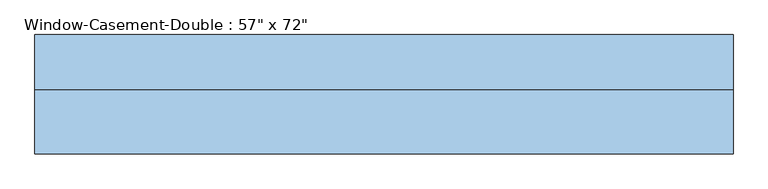
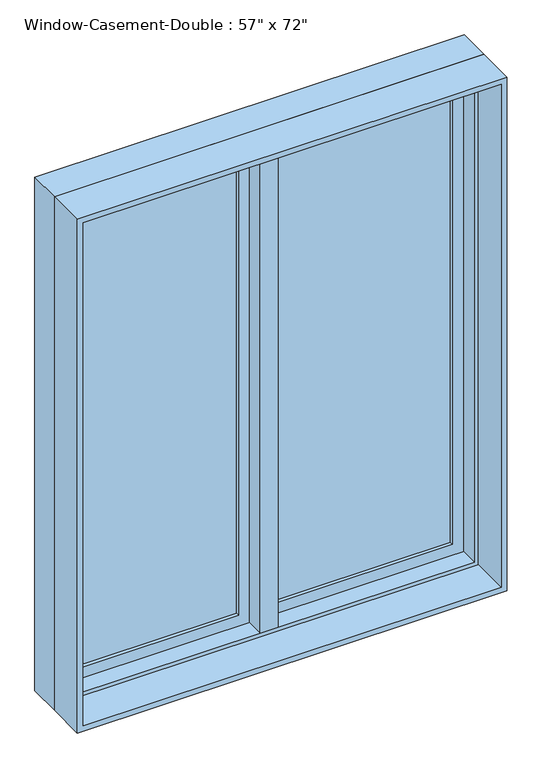
"""IFC4 building model written with IfcOpenShell, lengths in millimetres: window geometry."""

from ifc_helpers import new_model, si_unit, frame, origin, place, context, project, spatial, polyline, outline, extrude, faceted_brep, source, transform, mapped, element, save


def window_9ac97e1a(model_context):
    return source(origin(), model_context, "Body", "SolidModel", [
        faceted_brep([(9.525, 133.35, 2730.5), (-9.525, 133.35, 2730.5), (-9.525, 82.55, 2730.5), (9.525, 82.55, 2730.5), (9.525, 133.35, 927.1), (9.525, 82.55, 927.1), (-9.525, 82.55, 927.1), (-9.525, 133.35, 927.1), (-9.525, 82.55, 946.15), (-9.525, 82.55, 2711.45), (-30.1625, 82.55, 946.15), (-30.1625, 82.55, 2711.45), (-30.1625, 19.05, 946.15), (-30.1625, 19.05, 2711.45), (30.1625, 19.05, 946.15), (30.1625, 19.05, 2711.45), (30.1625, 82.55, 946.15), (30.1625, 82.55, 2711.45), (9.525, 82.55, 946.15), (9.525, 82.55, 2711.45)], [[[0, 1, 2, 3]], [[4, 5, 6, 7]], [[1, 0, 4, 7]], [[2, 1, 7, 6, 8, 9]], [[9, 8, 10, 11]], [[11, 10, 12, 13]], [[13, 12, 14, 15]], [[15, 14, 16, 17]], [[17, 16, 18, 19]], [[0, 3, 19, 18, 5, 4]], [[18, 8, 6, 5]], [[9, 19, 3, 2]], [[8, 18, 16, 14, 12, 10]], [[19, 9, 11, 13, 15, 17]]]),
        extrude(outline(polyline([(-66.675, 114.3), (-66.675, 107.95), (-654.05, 107.95), (-654.05, 114.3), (-66.675, 114.3)])), frame((0.0, 0.0, 984.25), z_axis=(0.0, 0.0, 1.0), x_axis=(1.0, 0.0, 0.0)), (0.0, 0.0, 1.0), 1689.1),
        extrude(outline(polyline([(-654.05, 95.25), (-654.05, 101.6), (-66.675, 101.6), (-66.675, 95.25), (-654.05, 95.25)])), frame((0.0, 0.0, 984.25), z_axis=(0.0, 0.0, 1.0), x_axis=(1.0, 0.0, 0.0)), (0.0, 0.0, 1.0), 1689.1),
        extrude(outline(polyline([(654.05, 114.3), (654.05, 107.95), (66.675, 107.95), (66.675, 114.3), (654.05, 114.3)])), frame((0.0, 0.0, 984.25), z_axis=(0.0, 0.0, 1.0), x_axis=(1.0, 0.0, 0.0)), (0.0, 0.0, 1.0), 1689.1),
        extrude(outline(polyline([(66.675, 95.25), (66.675, 101.6), (654.05, 101.6), (654.05, 95.25), (66.675, 95.25)])), frame((0.0, 0.0, 984.25), z_axis=(0.0, 0.0, 1.0), x_axis=(1.0, 0.0, 0.0)), (0.0, 0.0, 1.0), 1689.1),
        extrude(outline(polyline([(2730.5, -711.2), (927.1, -711.2), (927.1, -9.525), (2730.5, -9.525), (2730.5, -711.2)]), holes=[polyline([(2673.35, -66.675), (984.25, -66.675), (984.25, -654.05), (2673.35, -654.05), (2673.35, -66.675)])]), frame((0.0, 82.55, 0.0), z_axis=(0.0, 1.0, 0.0), x_axis=(0.0, 0.0, 1.0)), (0.0, 0.0, 1.0), 44.45),
        extrude(outline(polyline([(927.1, 711.2), (2730.5, 711.2), (2730.5, 9.525), (927.1, 9.525), (927.1, 711.2)]), holes=[polyline([(984.25, 66.675), (2673.35, 66.675), (2673.35, 654.05), (984.25, 654.05), (984.25, 66.675)])]), frame((0.0, 82.55, 0.0), z_axis=(0.0, 1.0, 0.0), x_axis=(0.0, 0.0, 1.0)), (0.0, 0.0, 1.0), 44.45),
        extrude(outline(polyline([(2743.2, -723.9), (914.4, -723.9), (914.4, 723.9), (2743.2, 723.9), (2743.2, -723.9)]), holes=[polyline([(2724.15, 704.85), (933.45, 704.85), (933.45, -704.85), (2724.15, -704.85), (2724.15, 704.85)])]), frame((0.0, -114.3, 0.0), z_axis=(0.0, 1.0, 0.0), x_axis=(0.0, 0.0, 1.0)), (0.0, 0.0, 1.0), 133.35),
        faceted_brep([(692.15, 82.55, 2711.45), (692.15, 19.05, 2711.45), (-692.15, 19.05, 2711.45), (-692.15, 82.55, 2711.45), (711.2, 133.35, 2730.5), (711.2, 82.55, 2730.5), (-711.2, 82.55, 2730.5), (-711.2, 133.35, 2730.5), (723.9, 19.05, 2743.2), (723.9, 133.35, 2743.2), (-723.9, 133.35, 2743.2), (-723.9, 19.05, 2743.2), (-692.15, 19.05, 946.15), (-692.15, 82.55, 946.15), (-711.2, 82.55, 927.1), (-711.2, 133.35, 927.1), (-723.9, 133.35, 914.4), (-723.9, 19.05, 914.4), (692.15, 19.05, 946.15), (692.15, 82.55, 946.15), (711.2, 82.55, 927.1), (711.2, 133.35, 927.1), (723.9, 133.35, 914.4), (723.9, 19.05, 914.4)], [[[0, 1, 2, 3]], [[4, 5, 6, 7]], [[8, 9, 10, 11]], [[3, 2, 12, 13]], [[7, 6, 14, 15]], [[11, 10, 16, 17]], [[13, 12, 18, 19]], [[15, 14, 20, 21]], [[17, 16, 22, 23]], [[11, 17, 23, 8], [1, 18, 12, 2]], [[19, 18, 1, 0]], [[5, 20, 14, 6], [3, 13, 19, 0]], [[21, 20, 5, 4]], [[23, 22, 9, 8]], [[9, 22, 16, 10], [7, 15, 21, 4]]]),
    ])


if __name__ == "__main__":
    model = new_model("IFC4")
    model_context = context("Model", 3, world=origin())
    ifc_project = project(units=[si_unit("LENGTHUNIT", "METRE", prefix="MILLI")], contexts=[model_context])
    site = spatial("IfcSite", under=ifc_project)
    building = spatial("IfcBuilding", under=site)
    placement = place(None, origin())
    window_shape = window_9ac97e1a(model_context)
    element("IfcWindow", 1, ObjectType="Window-Casement-Double : 57\" x 72\"", at=placement, inside=building, context=model_context, shape_type="MappedRepresentation", body=[
        mapped(window_shape, transform((0.0, 0.0, 0.0), x_axis=(1.0, 0.0, 0.0), y_axis=(0.0, 1.0, 0.0), z_axis=(0.0, 0.0, 1.0))),
    ])
    save(model, "model.ifc")

# Revit data of these elements
# Type "Window-Casement-Double : 57\" x 72\""
#   Type Mark = "17"
#   Fire Rating = "0.5h"
#   Assembly Code = "B2020100"
#   Analytic Construction = "Double glazing - domestic"
#   Frame Extension [instance default] = 0' - 0 1/4"
#   Window Inset [instance default] = 0' - 0"
#   Wall Thickness [instance default] = 0' - 6"
#   Interior Wall Closure [instance default] = 0' - 2 1/4"
#   Half Width = 2' - 4 1/2"
#   Visual Light Transmittance = 0.81
#   Thermal Resistance (R) = 1.8146 (h·ft²·°F)/BTU
#   Solar Heat Gain Coefficient = 0.76
#   Rough Width = 4' - 9 1/2"
#   Rough Height = 6' - 0 1/2"
#   Height = 6' - 0"
#   Heat Transfer Coefficient (U) = 0.5511 BTU/(h·ft²·°F)
#   Exterior Wall Closure [instance default] = 0' - 1 1/4"
#   Extension Jamb [instance default] = 0' - 2 1/4"
#   Default Sill Height = 3' - 0"
#   Width = 4' - 9"
#   Define Thermal Properties by = 0
#   Muntin Visibility = yes
#   Interior Trim Visibility [instance default] = yes
#   Exterior Trim Visibility [instance default] = yes
#   Extension Jamb Visibility [instance default] = yes
#   Interior Trim Material = Wood - Stained
#   Muntin Pattern = Muntin Pattern_2x2 : Muntin Pattern_2x2
#   Interior Trim = Trim-Window-Interior-Flat : Picture Frame
#   Interior Frame Material = Wood - Stained
#   Glass Panel Material = Glass
#   Exterior Trim Material = Clad - White
#   Exterior Trim = Trim-Window-Exterior-Flat : with Sill
#   Exterior Frame Material = Clad - White
#   Wall Closure = (empty or 0)
# Element 1 (IfcWindow, "Window-Casement-Double : 57\" x 72\"")
#   Wall Thickness = 0' - 9"
#   Extension Jamb = 0' - 5 1/4"
#   Materials on its faces: "Wood - Stained", "Glass", "Clad - White"
# Materials
#   "Wood - Stained": class "Wood", colour RGB 224 178 126, transparency 0, Cost = 0
#   "Glass": class "Glass", colour RGB 0 128 192, transparency 0.75, Description = "Soda Lime Glass", Cost = 0
#   "Clad - White": class "Wood", colour RGB 242 242 238, transparency 0, Cost = 0
